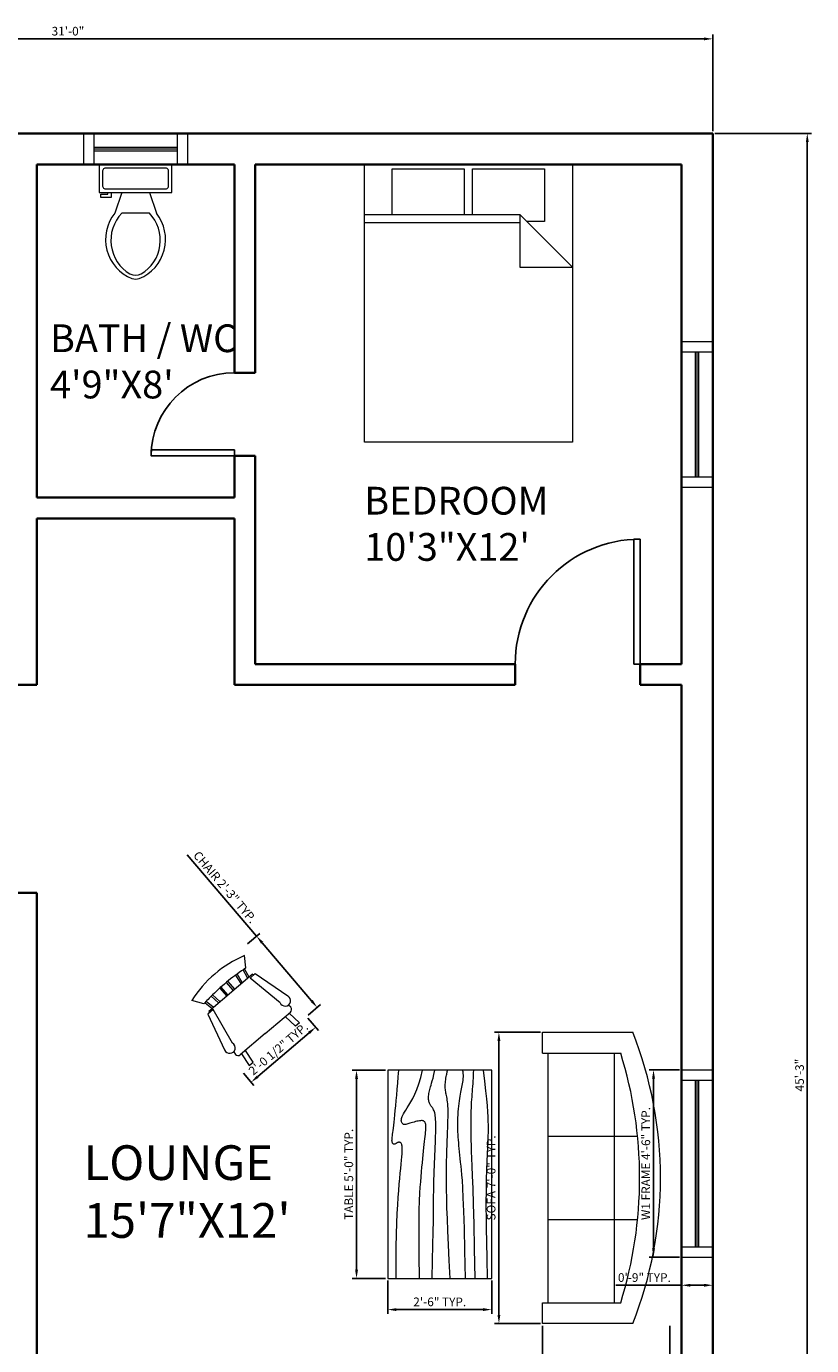
# Model space of a CAD drawing. Units: inches. Extents: x 2163 to 7246, y 928 to 2098.
# Tile 13 of 15: x 5407 to 5633, y 1651 to 2032. Entities that reach past the tile are written whole.
import ezdxf

# ---------------------------------------------------------------- set-up
doc = ezdxf.new("R2010")
doc.units = ezdxf.units.IN
for name, color, linetype, lineweight in [('A-ANNO-DIMS', 4, 'Continuous', 18), ('A-AREA-IDEN', 7, 'Continuous', 18), ('A-DOOR', 4, 'Continuous', 25), ('A-FLOR-FIXT', 9, 'Continuous', 20), ('A-FURN', 8, 'Continuous', 18), ('A-GLAZ', 30, 'Continuous', 20), ('A-WALL', 7, 'Continuous', 35)]:
    doc.layers.add(name, color=color, linetype=linetype, lineweight=lineweight)
doc.styles.get("Standard").update_dxf_attribs({"font": 'arial.ttf'})
doc.dimstyles.new('ISO-25', dxfattribs={"dimtxt": 2.5, "dimasz": 2.5, "dimexe": 1.25, "dimexo": 0.625, "dimtad": 1, "dimdec": 0, "dimlunit": 3, "dimtxsty": 'Standard', "dimcen": 2.5, "dimadec": 0, "dimazin": 0, "dimtfac": 1, "dimtdec": 0, "dimtmove": 0, "dimatfit": 3, "dimfxl": 1, "dimarcsym": 0})

# ---------------------------------------------------------------- blocks, each defined once
blk = doc.blocks.new('*U30')
for p, q in [((0, 0), (0, -6)), ((-36, 0), (-36, -6))]:
    blk.add_line(p, q)
blk.add_lwpolyline([(0, 0), (0, 36), (-1.75, 36), (-1.75, 0)], close=True)
blk.add_arc((0, 0), 36, 90, 180)
blk = doc.blocks.new('*U34')
for p, q in [((-24, 0), (-24, 6)), ((0, 0), (0, 6))]:
    blk.add_line(p, q)
blk.add_lwpolyline([(0, 0), (0, -24), (-1.75, -24), (-1.75, 0)], close=True)
blk.add_arc((0, 0), 24, 180, 270)
blk = doc.blocks.new('Bed - Queen')
for p, q in [((0, -80.00003), (0, 0)), ((0, 0), (59.99999, 0)), ((59.99999, 0), (59.99999, -80.00003)), ((7.99999, -1.2), (28.79998, -1.2)), ((7.99999, -14.4), (7.99999, -1.2)), ((28.79998, -1.2), (28.79998, -14.4)), ((31.19999, -1.2), (51.99999, -1.2)), ((31.19999, -14.4), (31.19999, -1.2)), ((51.99999, -1.2), (51.99999, -16.4)), ((0, -14.4), (44.8, -14.4)), ((59.99999, -29.6), (44.8, -14.4)), ((44.8, -14.4), (44.8, -29.6)), ((44.8, -16.8), (0, -16.8)), ((51.99999, -16.4), (46.79936, -16.4)), ((44.8, -29.6), (59.99999, -29.6)), ((59.99999, -80.00003), (0, -80.00003))]:
    blk.add_line(p, q)
blk = doc.blocks.new('Toilet - top')
for p, q in [((9.5, -6), (9.5, -2)), ((-10, -8.5), (-8, -8.5)), ((-10, -9.5), (-10, -8.5)), ((-7, -9.5), (-10, -9.5)), ((-8, -8.5), (-8, -8)), ((-7, -8), (-7, -9.5)), ((-4, -8), (-6, -14)), ((4, -8), (6, -14)), ((4, -14), (-4, -14))]:
    blk.add_line(p, q)
blk.add_lwpolyline([(10.5, -8), (10.5, 0), (-10.5, 0), (-10.5, -8)], close=True)
for points in [[(-9.5, -2), (-9.5, -6)], [(8.5, -1), (-8.5, -1)], [(-8.5, -7), (8.5, -7)]]:
    blk.add_lwpolyline(points)
for centre, radius, start, end in [((-8.62, -1.88), 0.884, 81.8699, 188.1301), ((8.62, -1.88), 0.884, 351.8699, 98.1301), ((-8.62, -6.12), 0.884, 171.8699, 278.1301), ((8.62, -6.12), 0.884, 261.8699, 8.1301), ((3.52, -21.58), 12.17, 141.4691, 247.9714), ((4.2, -21.82), 11.33, 136.3677, 238.9468), ((-3.52, -21.58), 12.17, 292.0284, 38.5307), ((-4.2, -21.82), 11.33, 301.053, 43.6321), ((0, -27.88), 4, 245.7318, 294.2682), ((0, -29), 4, 254.8605, 285.1395)]:
    blk.add_arc(centre, radius, start, end)
blk = doc.blocks.new('Sofa - Roundback 7 ft.')
for p, q in [((-12.00002, -32.4421), (-12.00003, -6.5971)), ((11.99997, -32.4421), (11.99998, -6.5971)), ((-36.000027, -34), (-36.000027, -11.4696)), ((-35.999844, -13.3819), (35.9998, -13.3819)), ((35.99998, -34), (35.99998, -11.4696)), ((-36.000027, -32.4421), (35.99998, -32.4421))]:
    blk.add_line(p, q)
for points in [[(-36.000027, -34), (-42.000027, -34), (-42.000027, -8)], [(41.99998, -8), (41.99998, -34), (35.99998, -34)]]:
    blk.add_lwpolyline(points)
for centre, radius, start, end in [((0, -114.25), 114.25, 68.43141, 111.5686), ((-0.00001, -127.1968), 121.1968, 72.72033, 107.2797)]:
    blk.add_arc(centre, radius, start, end)
blk = doc.blocks.new('Chair - Rocking')
for p, q in [((-8, -4.5), (-10, -1.5)), ((8, -4.5), (10, -1.5)), ((-9, -7.5), (-12, -18.49999)), ((-7, -7.5), (-9, -7.5)), ((-9, -18.49999), (-7, -7.5)), ((-8.23428, -6.99939), (-8.3093, -7.47958)), ((-8.23041, -7), (8.23915, -7)), ((-7.5, -4.5), (-7, -7)), ((-6.5, -7), (-7.02225, -4.43)), ((-4.5, -7), (-4.96674, -4.19951)), ((-4, -7), (-4.40532, -4.16272)), ((-1.5, -4.05012), (-1.5, -7)), ((-1, -7), (-1, -4.05012)), ((1, -7), (1, -4.04655)), ((1.5, -4.05012), (1.5, -7)), ((4, -7), (4.40187, -4.18694)), ((4.5, -7), (4.96761, -4.19437)), ((6.5, -7), (7, -4.4057)), ((7.5, -4.5), (7, -7)), ((7, -7.5), (9, -7.5)), ((9, -18.49999), (7, -7.5)), ((8.31071, -7.48854), (8.23449, -7.00073)), ((9, -7.5), (12, -18.49999)), ((-10.36644, -20.64523), (-10.5, -21.49999)), ((-9, -22.49999), (-9.5, -26.49999)), ((0, -22.49999), (-9.5, -22.49999)), ((-8, -26.49999), (-7.5, -22.49999)), ((0, -22.49999), (9.5, -22.49999)), ((8, -26.49999), (7.5, -22.49999)), ((9, -22.49999), (9.5, -26.49999)), ((10.5, -21.49999), (10.3575, -20.58798)), ((-9.5, -26.49999), (-8, -26.49999)), ((9.5, -26.49999), (8, -26.49999))]:
    blk.add_line(p, q)
for centre, radius, start, end in [((0, -34.08333), 34.08333, 72.93847, 107.0615), ((0, -68.25004), 64.25, 93.92211, 97.15267), ((0, -68.25004), 64.25, 82.84733, 93.92211), ((-10.5, -18.99999), 1.58114, 161.5651, 18.43495), ((10.5, -18.99999), 1.58114, 161.5651, 18.43495), ((-9.5, -21.49999), 1, 180, 270), ((9.5, -21.49999), 1, 270, 0)]:
    blk.add_arc(centre, radius, start, end)
blk = doc.blocks.new('Table - Rectangular Woodgrain 60 x 30 in.')
for p, q in [((0, 0), (0, -30)), ((60, 0), (0, 0)), ((60, -30), (60, 0)), ((0, -30), (60, -30))]:
    blk.add_line(p, q)
for points in [[(0, -2.4), (4.8155, -2.418), (9.0302, -2.4688), (12.709, -2.5477), (15.9167, -2.65), (18.7181, -2.7711), (21.1781, -2.9063), (23.3616, -3.0508), (25.3333, -3.2), (27.1477, -3.3495), (28.8172, -3.4958), (30.3437, -3.636), (31.7291, -3.7667), (32.9756, -3.8849), (34.0849, -3.9875), (35.059, -4.0714), (35.9, -4.1334), (36.6114, -4.1711), (37.2041, -4.1854), (37.6906, -4.1779), (38.0833, -4.15), (38.3948, -4.1034), (38.6375, -4.0396), (38.8239, -3.9602), (38.9666, -3.8667), (39.0764, -3.7608), (39.1573, -3.6448), (39.2116, -3.521), (39.2416, -3.3917), (39.2498, -3.2593), (39.2385, -3.1261), (39.21, -2.9944), (39.1666, -2.8667), (39.111, -2.7447), (39.0468, -2.6281), (38.978, -2.5163), (38.9083, -2.4083), (38.8418, -2.3035), (38.7823, -2.201), (38.7337, -2.1001), (38.7, -2), (38.6844, -1.9003), (38.6875, -1.8021), (38.7094, -1.707), (38.75, -1.6167), (38.8094, -1.5326), (38.8875, -1.4563), (38.9844, -1.3893), (39.1, -1.3333), (39.2351, -1.2896), (39.3937, -1.2583), (39.5804, -1.2396), (39.8, -1.2333), (40.057, -1.2396), (40.3562, -1.2583), (40.7023, -1.2896), (41.1, -1.3333), (41.5547, -1.3895), (42.0755, -1.4573), (42.6721, -1.5361), (43.3542, -1.625), (44.1316, -1.7233), (45.014, -1.8302), (46.0114, -1.9449), (47.1333, -2.0667), (48.3862, -2.1947), (49.7625, -2.3281), (51.2513, -2.4663), (52.8416, -2.6083), (54.5226, -2.7535), (56.2833, -2.9011), (58.1127, -3.0501), (60, -3.2)], [(0, -9.2), (6.5759, -9.0858), (11.9385, -9.0365), (16.2527, -9.0418), (19.6833, -9.0917), (22.3952, -9.1759), (24.5531, -9.2844), (26.322, -9.4069), (27.8666, -9.5333), (29.3241, -9.6553), (30.7203, -9.7719), (32.0532, -9.8837), (33.3208, -9.9917), (34.5213, -10.0965), (35.6526, -10.199), (36.7128, -10.2999), (37.7, -10.4), (38.6129, -10.4996), (39.4531, -10.5969), (40.223, -10.6895), (40.925, -10.775), (41.5613, -10.8512), (42.1344, -10.9156), (42.6465, -10.966), (43.1, -11), (43.4976, -11.0158), (43.8437, -11.0136), (44.143, -10.9942), (44.4, -10.9583), (44.6195, -10.9069), (44.8062, -10.8406), (44.9648, -10.7603), (45.1, -10.6667), (45.2155, -10.5598), (45.3114, -10.4365), (45.3871, -10.2929), (45.4416, -10.125), (45.4743, -9.929), (45.4844, -9.7011), (45.4709, -9.4371), (45.4333, -9.1333), (45.3716, -8.7883), (45.2896, -8.4104), (45.1919, -8.0107), (45.0833, -7.6), (44.9685, -7.1893), (44.8521, -6.7896), (44.7388, -6.4117), (44.6333, -6.0667), (44.54, -5.7628), (44.4614, -5.4979), (44.4001, -5.2675), (44.3583, -5.0667), (44.3384, -4.8909), (44.3427, -4.7354), (44.3736, -4.5956), (44.4333, -4.4667), (44.5236, -4.3453), (44.6427, -4.2333), (44.7884, -4.1339), (44.9583, -4.05), (45.1501, -3.9849), (45.3614, -3.9417), (45.59, -3.9234), (45.8333, -3.9333), (46.0915, -3.9749), (46.3734, -4.0531), (46.6906, -4.1736), (47.0542, -4.3417), (47.4756, -4.5629), (47.9661, -4.8427), (48.5372, -5.1866), (49.2, -5.6), (49.9676, -6.0844), (50.8594, -6.625), (51.8965, -7.2031), (53.1, -7.8), (54.491, -8.3969), (56.0906, -8.975), (57.9199, -9.5156), (60, -10)], [(0, -12.8), (5.1847, -12.9322), (9.6213, -13.0323), (13.3963, -13.1059), (16.5958, -13.1583), (19.3063, -13.1952), (21.614, -13.2219), (23.6054, -13.2439), (25.3666, -13.2667), (26.9728, -13.2947), (28.4531, -13.3281), (29.8256, -13.3663), (31.1083, -13.4083), (32.3191, -13.4535), (33.476, -13.501), (34.597, -13.5501), (35.7, -13.6), (36.7984, -13.6497), (37.8875, -13.6979), (38.9578, -13.743), (40, -13.7833), (41.0047, -13.8174), (41.9625, -13.8438), (42.864, -13.8607), (43.7, -13.8667), (44.4631, -13.8604), (45.1552, -13.8417), (45.7801, -13.8104), (46.3416, -13.7667), (46.8439, -13.7104), (47.2906, -13.6417), (47.6858, -13.5604), (48.0333, -13.4667), (48.3375, -13.3608), (48.6042, -13.2448), (48.8396, -13.121), (49.05, -12.9917), (49.2417, -12.8593), (49.4208, -12.7261), (49.5937, -12.5944), (49.7667, -12.4667), (49.9452, -12.3451), (50.1323, -12.2313), (50.3303, -12.1268), (50.5416, -12.0333), (50.7686, -11.9524), (51.0135, -11.8854), (51.2788, -11.8341), (51.5666, -11.8), (51.8785, -11.7843), (52.2116, -11.7865), (52.562, -11.8059), (52.926, -11.8417), (53.2998, -11.8931), (53.6795, -11.9594), (54.0614, -12.0397), (54.4416, -12.1333), (54.8223, -12.2401), (55.2293, -12.3625), (55.6942, -12.5037), (56.2489, -12.6667), (56.9251, -12.8547), (57.7545, -13.0708), (58.7689, -13.3182), (60, -13.6)], [(0, -18), (5.124, -17.7273), (9.6609, -17.5057), (13.6705, -17.3303), (17.2125, -17.1958), (20.3467, -17.0973), (23.1328, -17.0297), (25.6307, -16.9878), (27.9, -16.9667), (29.9928, -16.9617), (31.9302, -16.9703), (33.7254, -16.9907), (35.3917, -17.0208), (36.9423, -17.0588), (38.3906, -17.1026), (39.7499, -17.1503), (41.0333, -17.2), (42.2519, -17.2496), (43.4073, -17.2969), (44.4986, -17.3395), (45.525, -17.375), (46.4858, -17.4012), (47.3802, -17.4156), (48.2074, -17.416), (48.9667, -17.4), (49.6583, -17.3662), (50.2872, -17.3167), (50.8595, -17.2547), (51.3812, -17.1833), (51.8584, -17.1057), (52.2971, -17.025), (52.7034, -16.9443), (53.0833, -16.8667), (53.443, -16.7951), (53.789, -16.7313), (54.128, -16.6768), (54.4666, -16.6334), (54.8115, -16.6024), (55.1693, -16.5854), (55.5465, -16.5841), (55.95, -16.6), (56.3828, -16.6337), (56.8346, -16.6823), (57.2915, -16.7418), (57.7396, -16.8084), (58.165, -16.878), (58.5539, -16.9469), (58.8924, -17.0111), (59.1666, -17.0667), (59.3679, -17.1107), (59.5078, -17.1438), (59.6032, -17.1675), (59.6708, -17.1833), (59.7275, -17.193), (59.7901, -17.1979), (59.8753, -17.1998), (60, -17.2)], [(0, -22.4), (8.0098, -22.2501), (14.4094, -22.1011), (19.4168, -21.9535), (23.25, -21.8083), (26.1269, -21.6663), (28.2656, -21.5281), (29.884, -21.3947), (31.2, -21.2667), (32.3967, -21.1448), (33.5172, -21.0292), (34.5697, -20.9198), (35.5625, -20.8167), (36.5037, -20.7198), (37.4015, -20.6292), (38.2642, -20.5448), (39.1, -20.4667), (39.9164, -20.3951), (40.7187, -20.3313), (41.5117, -20.2768), (42.3, -20.2333), (43.0883, -20.2024), (43.8812, -20.1854), (44.6836, -20.1841), (45.5, -20.2), (46.3328, -20.234), (47.1747, -20.2844), (48.0163, -20.3488), (48.8479, -20.425), (49.66, -20.5106), (50.4429, -20.6031), (51.1872, -20.7004), (51.8833, -20.8), (52.5246, -20.8999), (53.1166, -20.9995), (53.6681, -21.0983), (54.1875, -21.1958), (54.6834, -21.2919), (55.1646, -21.3859), (55.6394, -21.4777), (56.1167, -21.5667), (56.6028, -21.6515), (57.0961, -21.7266), (57.5929, -21.7852), (58.0896, -21.8208), (58.5823, -21.8268), (59.0674, -21.7964), (59.5412, -21.723), (60, -21.6)], [(0, -25.2), (8.6355, -25.0504), (15.7026, -24.9031), (21.4049, -24.7606), (25.9458, -24.625), (29.529, -24.4988), (32.3578, -24.3844), (34.6359, -24.284), (36.5667, -24.2), (38.3213, -24.1341), (39.9417, -24.0854), (41.437, -24.0523), (42.8167, -24.0333), (44.0901, -24.0268), (45.2667, -24.0313), (46.3557, -24.0451), (47.3667, -24.0667), (48.309, -24.0947), (49.1928, -24.1287), (50.0284, -24.168), (50.826, -24.2125), (51.5959, -24.2617), (52.3483, -24.3151), (53.0935, -24.3725), (53.8417, -24.4334), (54.6009, -24.497), (55.3699, -24.561), (56.1454, -24.6226), (56.9239, -24.6792), (57.7021, -24.7279), (58.4764, -24.7662), (59.2435, -24.7911), (60, -24.8)], [(0, -28.8), (5.6867, -28.6681), (10.45, -28.5698), (14.407, -28.5012), (17.675, -28.4584), (20.3711, -28.4374), (22.6125, -28.4344), (24.5164, -28.4455), (26.2, -28.4667), (27.762, -28.4947), (29.2276, -28.5281), (30.6033, -28.5663), (31.8958, -28.6084), (33.1118, -28.6535), (34.2578, -28.7011), (35.3405, -28.7501), (36.3666, -28.8), (37.3443, -28.8497), (38.288, -28.8974), (39.2137, -28.9412), (40.1375, -28.9792), (41.0753, -29.0093), (42.0432, -29.0297), (43.0572, -29.0384), (44.1333, -29.0333), (45.2936, -29.0114), (46.5843, -28.9641), (48.0579, -28.8816), (49.7666, -28.7542), (51.7629, -28.5721), (54.0989, -28.3255), (56.8272, -28.0048), (60, -27.6)]]:
    blk.add_lwpolyline(points)
blk = doc.blocks.new('WIN-36-PLAN')
for p, q in [((0, 9), (0, 0)), ((3, 9), (3, 0)), ((39, 9), (39, 0)), ((42, 9), (42, 0)), ((3, 5), (39, 5)), ((3, 4.5), (39, 4.5)), ((3, 4), (39, 4))]:
    blk.add_line(p, q)
blk = doc.blocks.new('VENT-24-PLAN')
for p, q in [((9, 30), (0, 30)), ((9, 27), (0, 27)), ((4, 27), (4, 3)), ((4.5, 27), (4.5, 3)), ((5, 27), (5, 3)), ((9, 3), (0, 3)), ((9, 0), (0, 0))]:
    blk.add_line(p, q)
blk = doc.blocks.new('WIN-48-PLAN')
for p, q in [((0, 9), (0, 0)), ((3, 9), (3, 0)), ((51, 9), (51, 0)), ((54, 9), (54, 0)), ((3, 5), (51, 5)), ((3, 4.5), (51, 4.5)), ((3, 4), (51, 4))]:
    blk.add_line(p, q)
blk = doc.blocks.new('TABLE-60X30-GRAIN')
for p, q in [((0, 30), (0, 0)), ((60, 30), (0, 30)), ((60, 0), (60, 30)), ((0, 0), (60, 0))]:
    blk.add_line(p, q)
for points in [[(0, 27.6), (4.8155, 27.582), (9.0302, 27.5312), (12.709, 27.4523), (15.9167, 27.35), (18.7181, 27.2289), (21.1781, 27.0937), (23.3616, 26.9492), (25.3333, 26.8), (27.1477, 26.6505), (28.8172, 26.5042), (30.3437, 26.364), (31.7291, 26.2333), (32.9756, 26.1151), (34.0849, 26.0125), (35.059, 25.9286), (35.9, 25.8666), (36.6114, 25.8289), (37.2041, 25.8146), (37.6906, 25.8221), (38.0833, 25.85), (38.3948, 25.8966), (38.6375, 25.9604), (38.8239, 26.0398), (38.9666, 26.1333), (39.0764, 26.2392), (39.1573, 26.3552), (39.2116, 26.479), (39.2416, 26.6083), (39.2498, 26.7407), (39.2385, 26.8739), (39.21, 27.0056), (39.1666, 27.1333), (39.111, 27.2553), (39.0468, 27.3719), (38.978, 27.4837), (38.9083, 27.5917), (38.8418, 27.6965), (38.7823, 27.799), (38.7337, 27.8999), (38.7, 28), (38.6844, 28.0997), (38.6875, 28.1979), (38.7094, 28.293), (38.75, 28.3833), (38.8094, 28.4674), (38.8875, 28.5437), (38.9844, 28.6107), (39.1, 28.6667), (39.2351, 28.7104), (39.3937, 28.7417), (39.5804, 28.7604), (39.8, 28.7667), (40.057, 28.7604), (40.3562, 28.7417), (40.7023, 28.7104), (41.1, 28.6667), (41.5547, 28.6105), (42.0755, 28.5427), (42.6721, 28.4639), (43.3542, 28.375), (44.1316, 28.2767), (45.014, 28.1698), (46.0114, 28.0551), (47.1333, 27.9333), (48.3862, 27.8053), (49.7625, 27.6719), (51.2513, 27.5337), (52.8416, 27.3917), (54.5226, 27.2465), (56.2833, 27.0989), (58.1127, 26.9499), (60, 26.8)], [(0, 20.8), (6.5759, 20.9142), (11.9385, 20.9635), (16.2527, 20.9582), (19.6833, 20.9083), (22.3952, 20.8241), (24.5531, 20.7156), (26.322, 20.5931), (27.8666, 20.4667), (29.3241, 20.3447), (30.7203, 20.2281), (32.0532, 20.1163), (33.3208, 20.0083), (34.5213, 19.9035), (35.6526, 19.801), (36.7128, 19.7001), (37.7, 19.6), (38.6129, 19.5004), (39.4531, 19.4031), (40.223, 19.3105), (40.925, 19.225), (41.5613, 19.1488), (42.1344, 19.0844), (42.6465, 19.034), (43.1, 19), (43.4976, 18.9842), (43.8437, 18.9864), (44.143, 19.0058), (44.4, 19.0417), (44.6195, 19.0931), (44.8062, 19.1594), (44.9648, 19.2397), (45.1, 19.3333), (45.2155, 19.4402), (45.3114, 19.5635), (45.3871, 19.7071), (45.4416, 19.875), (45.4743, 20.071), (45.4844, 20.2989), (45.4709, 20.5629), (45.4333, 20.8667), (45.3716, 21.2117), (45.2896, 21.5896), (45.1919, 21.9893), (45.0833, 22.4), (44.9685, 22.8107), (44.8521, 23.2104), (44.7388, 23.5883), (44.6333, 23.9333), (44.54, 24.2372), (44.4614, 24.5021), (44.4001, 24.7325), (44.3583, 24.9333), (44.3384, 25.1091), (44.3427, 25.2646), (44.3736, 25.4044), (44.4333, 25.5333), (44.5236, 25.6547), (44.6427, 25.7667), (44.7884, 25.8661), (44.9583, 25.95), (45.1501, 26.0151), (45.3614, 26.0583), (45.59, 26.0766), (45.8333, 26.0667), (46.0915, 26.0251), (46.3734, 25.9469), (46.6906, 25.8264), (47.0542, 25.6583), (47.4756, 25.4371), (47.9661, 25.1573), (48.5372, 24.8134), (49.2, 24.4), (49.9676, 23.9156), (50.8594, 23.375), (51.8965, 22.7969), (53.1, 22.2), (54.491, 21.6031), (56.0906, 21.025), (57.9199, 20.4844), (60, 20)], [(0, 17.2), (5.1847, 17.0678), (9.6213, 16.9677), (13.3963, 16.8941), (16.5958, 16.8417), (19.3063, 16.8048), (21.614, 16.7781), (23.6054, 16.7561), (25.3666, 16.7333), (26.9728, 16.7053), (28.4531, 16.6719), (29.8256, 16.6337), (31.1083, 16.5917), (32.3191, 16.5465), (33.476, 16.499), (34.597, 16.4499), (35.7, 16.4), (36.7984, 16.3503), (37.8875, 16.3021), (38.9578, 16.257), (40, 16.2167), (41.0047, 16.1826), (41.9625, 16.1562), (42.864, 16.1393), (43.7, 16.1333), (44.4631, 16.1396), (45.1552, 16.1583), (45.7801, 16.1896), (46.3416, 16.2333), (46.8439, 16.2896), (47.2906, 16.3583), (47.6858, 16.4396), (48.0333, 16.5333), (48.3375, 16.6392), (48.6042, 16.7552), (48.8396, 16.879), (49.05, 17.0083), (49.2417, 17.1407), (49.4208, 17.2739), (49.5937, 17.4056), (49.7667, 17.5333), (49.9452, 17.6549), (50.1323, 17.7687), (50.3303, 17.8732), (50.5416, 17.9667), (50.7686, 18.0476), (51.0135, 18.1146), (51.2788, 18.1659), (51.5666, 18.2), (51.8785, 18.2157), (52.2116, 18.2135), (52.562, 18.1941), (52.926, 18.1583), (53.2998, 18.1069), (53.6795, 18.0406), (54.0614, 17.9603), (54.4416, 17.8667), (54.8223, 17.7599), (55.2293, 17.6375), (55.6942, 17.4963), (56.2489, 17.3333), (56.9251, 17.1453), (57.7545, 16.9292), (58.7689, 16.6818), (60, 16.4)], [(0, 12), (5.124, 12.2727), (9.6609, 12.4943), (13.6705, 12.6697), (17.2125, 12.8042), (20.3467, 12.9027), (23.1328, 12.9703), (25.6307, 13.0122), (27.9, 13.0333), (29.9928, 13.0383), (31.9302, 13.0297), (33.7254, 13.0093), (35.3917, 12.9792), (36.9423, 12.9412), (38.3906, 12.8974), (39.7499, 12.8497), (41.0333, 12.8), (42.2519, 12.7504), (43.4073, 12.7031), (44.4986, 12.6605), (45.525, 12.625), (46.4858, 12.5988), (47.3802, 12.5844), (48.2074, 12.584), (48.9667, 12.6), (49.6583, 12.6338), (50.2872, 12.6833), (50.8595, 12.7453), (51.3812, 12.8167), (51.8584, 12.8943), (52.2971, 12.975), (52.7034, 13.0557), (53.0833, 13.1333), (53.443, 13.2049), (53.789, 13.2687), (54.128, 13.3232), (54.4666, 13.3666), (54.8115, 13.3976), (55.1693, 13.4146), (55.5465, 13.4159), (55.95, 13.4), (56.3828, 13.3663), (56.8346, 13.3177), (57.2915, 13.2582), (57.7396, 13.1916), (58.165, 13.122), (58.5539, 13.0531), (58.8924, 12.9889), (59.1666, 12.9333), (59.3679, 12.8893), (59.5078, 12.8562), (59.6032, 12.8325), (59.6708, 12.8167), (59.7275, 12.807), (59.7901, 12.8021), (59.8753, 12.8002), (60, 12.8)], [(0, 7.6), (8.0098, 7.7499), (14.4094, 7.8989), (19.4168, 8.0465), (23.25, 8.1917), (26.1269, 8.3337), (28.2656, 8.4719), (29.884, 8.6053), (31.2, 8.7333), (32.3967, 8.8552), (33.5172, 8.9708), (34.5697, 9.0802), (35.5625, 9.1833), (36.5037, 9.2802), (37.4015, 9.3708), (38.2642, 9.4552), (39.1, 9.5333), (39.9164, 9.6049), (40.7187, 9.6687), (41.5117, 9.7232), (42.3, 9.7667), (43.0883, 9.7976), (43.8812, 9.8146), (44.6836, 9.8159), (45.5, 9.8), (46.3328, 9.766), (47.1747, 9.7156), (48.0163, 9.6512), (48.8479, 9.575), (49.66, 9.4894), (50.4429, 9.3969), (51.1872, 9.2996), (51.8833, 9.2), (52.5246, 9.1001), (53.1166, 9.0005), (53.6681, 8.9017), (54.1875, 8.8042), (54.6834, 8.7081), (55.1646, 8.6141), (55.6394, 8.5223), (56.1167, 8.4333), (56.6028, 8.3485), (57.0961, 8.2734), (57.5929, 8.2148), (58.0896, 8.1792), (58.5823, 8.1732), (59.0674, 8.2036), (59.5412, 8.277), (60, 8.4)], [(0, 4.8), (8.6355, 4.9496), (15.7026, 5.0969), (21.4049, 5.2394), (25.9458, 5.375), (29.529, 5.5012), (32.3578, 5.6156), (34.6359, 5.716), (36.5667, 5.8), (38.3213, 5.8659), (39.9417, 5.9146), (41.437, 5.9477), (42.8167, 5.9667), (44.0901, 5.9732), (45.2667, 5.9687), (46.3557, 5.9549), (47.3667, 5.9333), (48.309, 5.9053), (49.1928, 5.8713), (50.0284, 5.832), (50.826, 5.7875), (51.5959, 5.7383), (52.3483, 5.6849), (53.0935, 5.6275), (53.8417, 5.5666), (54.6009, 5.503), (55.3699, 5.439), (56.1454, 5.3774), (56.9239, 5.3208), (57.7021, 5.2721), (58.4764, 5.2338), (59.2435, 5.2089), (60, 5.2)], [(0, 1.2), (5.6867, 1.3319), (10.45, 1.4302), (14.407, 1.4988), (17.675, 1.5416), (20.3711, 1.5626), (22.6125, 1.5656), (24.5164, 1.5545), (26.2, 1.5333), (27.762, 1.5053), (29.2276, 1.4719), (30.6033, 1.4337), (31.8958, 1.3916), (33.1118, 1.3465), (34.2578, 1.2989), (35.3405, 1.2499), (36.3666, 1.2), (37.3443, 1.1503), (38.288, 1.1026), (39.2137, 1.0588), (40.1375, 1.0208), (41.0753, 0.9907), (42.0432, 0.9703), (43.0572, 0.9616), (44.1333, 0.9667), (45.2936, 0.9886), (46.5843, 1.0359), (48.0579, 1.1184), (49.7666, 1.2458), (51.7629, 1.4279), (54.0989, 1.6745), (56.8272, 1.9952), (60, 2.4)]]:
    blk.add_lwpolyline(points)
blk = doc.blocks.new('*D51')
at = {"layer": 'A-ANNO-DIMS', "color": 0, "lineweight": -2, "transparency": 16777216}
for p, q in [((5595.1, 1730.96), (5586.37, 1730.96)), ((5587.62, 1679.46), (5587.62, 1728.46)), ((5595.1, 1676.96), (5586.37, 1676.96))]:
    blk.add_line(p, q, dxfattribs=at)
at = {"layer": 'A-ANNO-DIMS', "color": 0, "transparency": 16777216}
for points in [[(5587.21, 1728.46), (5588.04, 1728.46), (5587.62, 1730.96)], [(5587.21, 1679.46), (5588.04, 1679.46), (5587.62, 1676.96)]]:
    blk.add_solid(points, dxfattribs=at)
at = {"layer": 'Defpoints', "color": 0, "transparency": 16777216}
for p in [(5587.62, 1730.96), (5595.72, 1730.96), (5595.72, 1676.96)]:
    blk.add_point(p, dxfattribs=at)
at = {"layer": 'A-ANNO-DIMS', "color": 0, "transparency": 16777216, "insert": (5585.72, 1703.96), "char_height": 2.5, "attachment_point": 5, "rotation": 90}
blk.add_mtext('W1 FRAME 4\'-6" TYP.', dxfattribs=at)
blk = doc.blocks.new('*D52')
at = {"layer": 'A-ANNO-DIMS', "color": 0, "lineweight": -2, "transparency": 16777216}
for p, q in [((5595.72, 1676.33), (5595.72, 1667.61)), ((5604.72, 1676.33), (5604.72, 1667.61)), ((5595.72, 1668.86), (5576.73, 1668.86)), ((5602.22, 1668.86), (5598.22, 1668.86))]:
    blk.add_line(p, q, dxfattribs=at)
at = {"layer": 'A-ANNO-DIMS', "color": 0, "transparency": 16777216}
for points in [[(5598.22, 1669.27), (5598.22, 1668.44), (5595.72, 1668.86)], [(5602.22, 1669.27), (5602.22, 1668.44), (5604.72, 1668.86)]]:
    blk.add_solid(points, dxfattribs=at)
at = {"layer": 'Defpoints', "color": 0, "transparency": 16777216}
for p in [(5595.72, 1676.96), (5604.72, 1676.96), (5595.72, 1668.86)]:
    blk.add_point(p, dxfattribs=at)
at = {"layer": 'A-ANNO-DIMS', "color": 0, "transparency": 16777216, "insert": (5584.98, 1670.76), "char_height": 2.5, "attachment_point": 5}
blk.add_mtext('0\'-9" TYP.', dxfattribs=at)
blk = doc.blocks.new('*D63')
at = {"layer": 'A-ANNO-DIMS', "color": 0, "lineweight": -2, "transparency": 16777216}
for p, q in [((5555, 1741.8), (5541.77, 1741.8)), ((5543.02, 1739.3), (5543.02, 1660.3)), ((5555, 1657.8), (5541.77, 1657.8))]:
    blk.add_line(p, q, dxfattribs=at)
at = {"layer": 'A-ANNO-DIMS', "color": 0, "transparency": 16777216}
for points in [[(5542.61, 1739.3), (5543.44, 1739.3), (5543.02, 1741.8)], [(5542.61, 1660.3), (5543.44, 1660.3), (5543.02, 1657.8)]]:
    blk.add_solid(points, dxfattribs=at)
at = {"layer": 'Defpoints', "color": 0, "transparency": 16777216}
for p in [(5555.62, 1741.8), (5543.02, 1657.8), (5555.62, 1657.8)]:
    blk.add_point(p, dxfattribs=at)
at = {"layer": 'A-ANNO-DIMS', "color": 0, "transparency": 16777216, "insert": (5541.1, 1699.8), "char_height": 2.5, "attachment_point": 5, "rotation": 90}
blk.add_mtext('SOFA 7\'-0" TYP.', dxfattribs=at)
blk = doc.blocks.new('*D64')
at = {"layer": 'A-ANNO-DIMS', "color": 0, "lineweight": -2, "transparency": 16777216}
for p, q in [((5555.62, 1657.18), (5555.62, 1643.95)), ((5592.29, 1657.18), (5592.29, 1643.95)), ((5558.12, 1645.2), (5589.79, 1645.2))]:
    blk.add_line(p, q, dxfattribs=at)
at = {"layer": 'A-ANNO-DIMS', "color": 0, "transparency": 16777216}
for points in [[(5558.12, 1645.62), (5558.12, 1644.78), (5555.62, 1645.2)], [(5589.79, 1645.62), (5589.79, 1644.78), (5592.29, 1645.2)]]:
    blk.add_solid(points, dxfattribs=at)
at = {"layer": 'Defpoints', "color": 0, "transparency": 16777216}
for p in [(5555.62, 1657.8), (5592.29, 1657.8), (5592.29, 1645.2)]:
    blk.add_point(p, dxfattribs=at)
at = {"layer": 'A-ANNO-DIMS', "color": 0, "transparency": 16777216, "insert": (5573.96, 1647.12), "char_height": 2.5, "attachment_point": 5}
blk.add_mtext('3\'-0 1/2" TYP.', dxfattribs=at)
blk = doc.blocks.new('*D65')
at = {"layer": 'A-ANNO-DIMS', "color": 0, "lineweight": -2, "transparency": 16777216}
for p, q in [((5473.11, 1769.51), (5453.14, 1792.95)), ((5470.5, 1767.29), (5474.06, 1770.32)), ((5488.99, 1750.86), (5474.73, 1767.61)), ((5488.01, 1746.73), (5491.57, 1749.76))]:
    blk.add_line(p, q, dxfattribs=at)
at = {"layer": 'A-ANNO-DIMS', "color": 0, "transparency": 16777216}
for points in [[(5475.04, 1767.88), (5474.41, 1767.34), (5473.11, 1769.51)], [(5489.31, 1751.13), (5488.68, 1750.59), (5490.61, 1748.95)]]:
    blk.add_solid(points, dxfattribs=at)
at = {"layer": 'Defpoints', "color": 0, "transparency": 16777216}
for p in [(5473.11, 1769.51), (5470.02, 1766.88), (5487.53, 1746.33)]:
    blk.add_point(p, dxfattribs=at)
at = {"layer": 'A-ANNO-DIMS', "color": 0, "transparency": 16777216, "insert": (5463.77, 1783.43), "char_height": 2.5, "attachment_point": 5, "rotation": 310.4239}
blk.add_mtext('CHAIR 2\'-3" TYP.', dxfattribs=at)
blk = doc.blocks.new('*D66')
at = {"layer": 'A-ANNO-DIMS', "color": 0, "lineweight": -2, "transparency": 16777216}
for p, q in [((5487.94, 1745.85), (5490.97, 1742.29)), ((5473.46, 1729.02), (5488.25, 1741.62)), ((5469.33, 1730.01), (5472.37, 1726.45))]:
    blk.add_line(p, q, dxfattribs=at)
at = {"layer": 'A-ANNO-DIMS', "color": 0, "transparency": 16777216}
for points in [[(5487.98, 1741.94), (5488.52, 1741.31), (5490.16, 1743.24)], [(5473.19, 1729.34), (5473.73, 1728.7), (5471.55, 1727.4)]]:
    blk.add_solid(points, dxfattribs=at)
at = {"layer": 'Defpoints', "color": 0, "transparency": 16777216}
for p in [(5487.53, 1746.33), (5490.16, 1743.24), (5468.93, 1730.48)]:
    blk.add_point(p, dxfattribs=at)
at = {"layer": 'A-ANNO-DIMS', "color": 0, "transparency": 16777216, "insert": (5479.61, 1736.78), "char_height": 2.5, "attachment_point": 5, "rotation": 40.4239}
blk.add_mtext('2\'-0 1/2" TYP.', dxfattribs=at)
blk = doc.blocks.new('*D67')
at = {"layer": 'A-ANNO-DIMS', "color": 0, "lineweight": -2, "transparency": 16777216}
for p, q in [((5510.33, 1730.84), (5500.7, 1730.84)), ((5501.95, 1673.34), (5501.95, 1728.34)), ((5510.33, 1670.84), (5500.7, 1670.84))]:
    blk.add_line(p, q, dxfattribs=at)
at = {"layer": 'A-ANNO-DIMS', "color": 0, "transparency": 16777216}
for points in [[(5501.54, 1728.34), (5502.37, 1728.34), (5501.95, 1730.84)], [(5501.54, 1673.34), (5502.37, 1673.34), (5501.95, 1670.84)]]:
    blk.add_solid(points, dxfattribs=at)
at = {"layer": 'Defpoints', "color": 0, "transparency": 16777216}
for p in [(5501.95, 1730.84), (5510.95, 1730.84), (5510.95, 1670.84)]:
    blk.add_point(p, dxfattribs=at)
at = {"layer": 'A-ANNO-DIMS', "color": 0, "transparency": 16777216, "insert": (5500.05, 1700.84), "char_height": 2.5, "attachment_point": 5, "rotation": 90}
blk.add_mtext('TABLE 5\'-0" TYP.', dxfattribs=at)
blk = doc.blocks.new('*D68')
at = {"layer": 'A-ANNO-DIMS', "color": 0, "lineweight": -2, "transparency": 16777216}
for p, q in [((5510.95, 1670.21), (5510.95, 1660.59)), ((5540.95, 1670.21), (5540.95, 1660.59)), ((5538.45, 1661.84), (5513.45, 1661.84))]:
    blk.add_line(p, q, dxfattribs=at)
at = {"layer": 'A-ANNO-DIMS', "color": 0, "transparency": 16777216}
for points in [[(5513.45, 1662.26), (5513.45, 1661.42), (5510.95, 1661.84)], [(5538.45, 1662.26), (5538.45, 1661.42), (5540.95, 1661.84)]]:
    blk.add_solid(points, dxfattribs=at)
at = {"layer": 'Defpoints', "color": 0, "transparency": 16777216}
for p in [(5510.95, 1670.84), (5540.95, 1670.84), (5510.95, 1661.84)]:
    blk.add_point(p, dxfattribs=at)
at = {"layer": 'A-ANNO-DIMS', "color": 0, "transparency": 16777216, "insert": (5525.95, 1663.74), "char_height": 2.5, "attachment_point": 5}
blk.add_mtext('2\'-6" TYP.', dxfattribs=at)
blk = doc.blocks.new('*D109')
at = {"layer": 'A-ANNO-DIMS', "color": 0, "lineweight": -2, "transparency": 16777216}
for p, q in [((5232.72, 2001.58), (5232.72, 2029.46)), ((5235.22, 2028.21), (5602.22, 2028.21)), ((5604.72, 2001.58), (5604.72, 2029.46))]:
    blk.add_line(p, q, dxfattribs=at)
at = {"layer": 'A-ANNO-DIMS', "color": 0, "transparency": 16777216}
for points in [[(5235.22, 2028.62), (5235.22, 2027.79), (5232.72, 2028.21)], [(5602.22, 2028.62), (5602.22, 2027.79), (5604.72, 2028.21)]]:
    blk.add_solid(points, dxfattribs=at)
at = {"layer": 'Defpoints', "color": 0, "transparency": 16777216}
for p in [(5604.72, 2028.21), (5232.72, 2000.96), (5604.72, 2000.96)]:
    blk.add_point(p, dxfattribs=at)
at = {"layer": 'A-ANNO-DIMS', "color": 0, "transparency": 16777216, "insert": (5418.72, 2030.11), "char_height": 2.5, "attachment_point": 5}
blk.add_mtext('31\'-0"', dxfattribs=at)
blk = doc.blocks.new('*D110')
at = {"layer": 'A-ANNO-DIMS', "color": 0, "lineweight": -2, "transparency": 16777216}
for p, q in [((5605.35, 2000.96), (5633.22, 2000.96)), ((5631.97, 1998.46), (5631.97, 1460.46)), ((5605.35, 1457.96), (5633.22, 1457.96))]:
    blk.add_line(p, q, dxfattribs=at)
at = {"layer": 'A-ANNO-DIMS', "color": 0, "transparency": 16777216}
for points in [[(5631.56, 1998.46), (5632.39, 1998.46), (5631.97, 2000.96)], [(5631.56, 1460.46), (5632.39, 1460.46), (5631.97, 1457.96)]]:
    blk.add_solid(points, dxfattribs=at)
at = {"layer": 'Defpoints', "color": 0, "transparency": 16777216}
for p in [(5604.72, 2000.96), (5604.72, 1457.96), (5631.97, 1457.96)]:
    blk.add_point(p, dxfattribs=at)
at = {"layer": 'A-ANNO-DIMS', "color": 0, "transparency": 16777216, "insert": (5630.07, 1729.46), "char_height": 2.5, "attachment_point": 5, "rotation": 90}
blk.add_mtext('45\'-3"', dxfattribs=at)

msp = doc.modelspace()

# ---------------------------------------------------------------- linework, layer by layer
at = {"layer": 'A-WALL'}
for p, q in [((5232.72, 2000.96), (5604.72, 2000.96)), ((5604.72, 2000.96), (5604.72, 1457.96)), ((5409.72, 1991.96), (5409.72, 1895.96)), ((5409.72, 1991.96), (5466.72, 1991.96)), ((5466.72, 1991.96), (5466.72, 1931.96)), ((5472.72, 1991.96), (5472.72, 1931.96)), ((5472.72, 1991.96), (5595.72, 1991.96)), ((5595.72, 1991.96), (5595.72, 1847.96)), ((5466.72, 1931.96), (5472.72, 1931.96)), ((5466.72, 1907.96), (5472.72, 1907.96)), ((5466.72, 1907.96), (5466.72, 1895.96)), ((5472.72, 1907.96), (5472.72, 1847.96)), ((5409.72, 1895.96), (5466.72, 1895.96)), ((5409.72, 1889.96), (5466.72, 1889.96)), ((5409.72, 1889.96), (5409.72, 1841.96)), ((5466.72, 1889.96), (5466.72, 1841.96)), ((5472.72, 1847.96), (5547.72, 1847.96)), ((5547.72, 1847.96), (5547.72, 1841.96)), ((5583.72, 1847.96), (5583.72, 1841.96)), ((5583.72, 1847.96), (5595.72, 1847.96)), ((5391.72, 1841.96), (5409.72, 1841.96)), ((5466.72, 1841.96), (5547.72, 1841.96)), ((5583.72, 1841.96), (5595.72, 1841.96)), ((5595.72, 1841.96), (5595.72, 1565.96)), ((5391.72, 1781.96), (5409.72, 1781.96)), ((5409.72, 1781.96), (5409.72, 1565.96))]:
    msp.add_line(p, q, dxfattribs=at)

# ---------------------------------------------------------------- block references
at = {"layer": 'A-DOOR', "rotation": 270}
msp.add_blockref('*U34', (5466.72, 1907.96), dxfattribs=at)
at = {"layer": 'A-DOOR'}
msp.add_blockref('*U30', (5583.72, 1847.96), dxfattribs=at)
at = {"layer": 'A-FLOR-FIXT'}
msp.add_blockref('Toilet - top', (5438.22, 1991.96), dxfattribs=at)
at = {"layer": 'A-FURN'}
msp.add_blockref('Bed - Queen', (5504.22, 1991.96), dxfattribs=at)
for name, p, rotation in [('Chair - Rocking', (5461.05, 1758.58), 40.42391738528442), ('Sofa - Roundback 7 ft.', (5589.62, 1699.8), 270), ('Table - Rectangular Woodgrain 60 x 30 in.', (5510.95, 1670.84), 90), ('TABLE-60X30-GRAIN', (5540.95, 1670.84), 90), ('TABLE-60X30-GRAIN', (5540.95, 1670.84), 90), ('TABLE-60X30-GRAIN', (5540.95, 1670.84), 90), ('TABLE-60X30-GRAIN', (5540.95, 1670.84), 90), ('TABLE-60X30-GRAIN', (5540.95, 1670.84), 90)]:
    msp.add_blockref(name, p, dxfattribs=dict(at, rotation=rotation))
at = {"layer": 'A-GLAZ', "rotation": 90}
for name, p in [('VENT-24-PLAN', (5453.22, 1991.96)), ('WIN-36-PLAN', (5604.72, 1898.96)), ('WIN-48-PLAN', (5604.72, 1676.96))]:
    msp.add_blockref(name, p, dxfattribs=at)

# ---------------------------------------------------------------- texts
at = {"layer": 'A-AREA-IDEN', "attachment_point": 1}
for s, width, insert, char_height in [('BATH / WC\\P4\'9"X8\'', 344.4804, (5413.55, 1945.89), 8), ('BEDROOM\\P10\'3"X12\'', 462.4335, (5504.19, 1899.06), 8), ('LOUNGE\\P15\'7"X12\'', 90.7352, (5423.21, 1709.21), 10)]:
    msp.add_mtext_dynamic_manual_height_columns(s, width=width, gutter_width=12.5, heights=[0], dxfattribs=dict(at, insert=insert, char_height=char_height))

# ---------------------------------------------------------------- dimensions: what is measured, and where the dimension line sits
at = {"layer": 'A-ANNO-DIMS'}
dim = msp.add_linear_dim(base=(5604.72, 2028.21), p1=(5232.72, 2000.96), p2=(5604.72, 2000.96), dimstyle='ISO-25', override={"dimdec": 1, "dimlfac": 1, "dimrnd": 0, "dimzin": 1, "dimdsep": 46, "dimlunit": 4, "dimfrac": 2}, dxfattribs=at)
dim.commit()
dim.dimension.update_dxf_attribs({"geometry": '*D109', "text_midpoint": (5418.72, 2030.11)})
dim = msp.add_linear_dim(base=(5631.97, 1457.96), p1=(5604.72, 2000.96), p2=(5604.72, 1457.96), angle=90, dimstyle='ISO-25', override={"dimdec": 1, "dimlfac": 1, "dimrnd": 0, "dimzin": 1, "dimdsep": 46, "dimlunit": 4, "dimfrac": 2}, dxfattribs=at)
dim.commit()
dim.dimension.update_dxf_attribs({"geometry": '*D110', "text_midpoint": (5630.07, 1729.46)})
for base, p1, p2, angle, text, picture, middle in [((5473.11, 1769.51), (5487.53, 1746.33), (5470.02, 1766.88), 130.4239, 'CHAIR <> TYP.', '*D65', (5463.77, 1783.43)), ((5490.16, 1743.24), (5468.93, 1730.48), (5487.53, 1746.33), 40.4239, '<> TYP.', '*D66', (5479.61, 1736.78)), ((5543.02, 1657.8), (5555.62, 1741.8), (5555.62, 1657.8), 270, 'SOFA <> TYP.', '*D63', (5541.1, 1699.8)), ((5501.95, 1730.84), (5510.95, 1670.84), (5510.95, 1730.84), 90, 'TABLE <> TYP.', '*D67', (5500.05, 1700.84)), ((5587.62, 1730.96), (5595.72, 1676.96), (5595.72, 1730.96), 90, 'W1 FRAME <> TYP.', '*D51', (5585.72, 1703.96)), ((5595.72, 1668.86), (5604.72, 1676.96), (5595.72, 1676.96), 180, '<> TYP.', '*D52', (5584.98, 1670.76)), ((5510.95, 1661.84), (5540.95, 1670.84), (5510.95, 1670.84), 180, '<> TYP.', '*D68', (5525.95, 1663.74))]:
    dim = msp.add_linear_dim(base=base, p1=p1, p2=p2, angle=angle, text=text, dimstyle='ISO-25', override={"dimdec": 1, "dimlfac": 1, "dimrnd": 0, "dimzin": 1, "dimdsep": 46, "dimlunit": 4, "dimfrac": 2}, dxfattribs=at)
    dim.commit()
    dim.dimension.update_dxf_attribs({"geometry": picture, "text_midpoint": middle})
dim = msp.add_linear_dim(base=(5592.29, 1645.2), p1=(5555.62, 1657.8), p2=(5592.29, 1657.8), text='<> TYP.', dimstyle='ISO-25', override={"dimdec": 1, "dimlfac": 1, "dimrnd": 0, "dimzin": 1, "dimdsep": 46, "dimlunit": 4, "dimfrac": 2}, dxfattribs=at)
dim.commit()
dim.dimension.update_dxf_attribs({"geometry": '*D64', "text_midpoint": (5573.96, 1647.12)})

doc.saveas('drawing.dxf')
